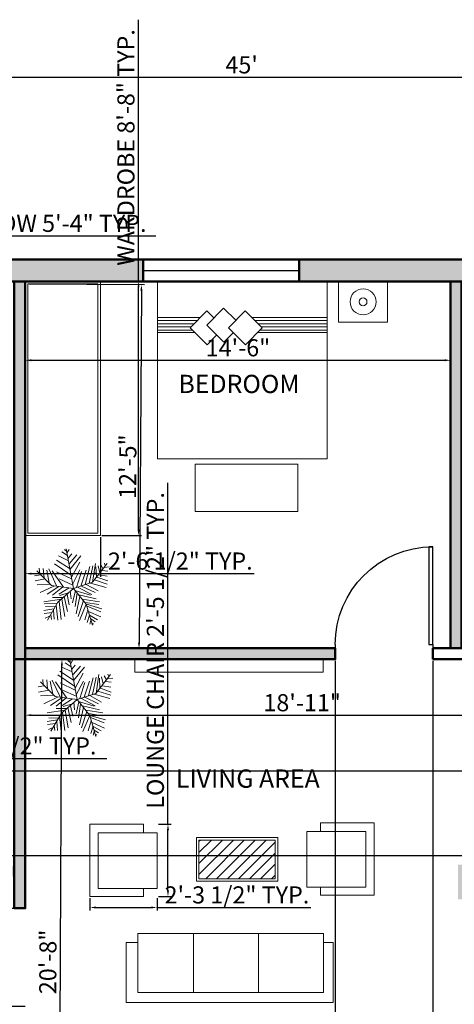
# Model space of a CAD drawing. Units: inches. Extents: x 1647 to 2354, y 1705 to 2321.
# Tile 3 of 4: x 1907 to 2085, y 1919 to 2321. Entities that reach past the tile are written whole.
import ezdxf

# ---------------------------------------------------------------- set-up
doc = ezdxf.new("R2010")
doc.units = ezdxf.units.IN
for name, color, linetype, lineweight in [('A-ANNO-DIMS', 130, 'Continuous', 18), ('A-AREA-IDEN', 7, 'Continuous', 25), ('A-FURN-PATT', 52, 'Continuous', 13), ('A-WALL-PATT', 84, 'Continuous', 13), ('door', 142, 'Continuous', 25), ('fur', 52, 'Continuous', 18), ('tree', 92, 'Continuous', 13), ('wall', 84, 'Continuous', 50), ('window', 242, 'Continuous', 25)]:
    doc.layers.add(name, color=color, linetype=linetype, lineweight=lineweight)
doc.styles.get("Standard").update_dxf_attribs({"font": 'arial.ttf'})
doc.dimstyles.new('ISO-25', dxfattribs={"dimtxt": 7, "dimasz": 2.5, "dimexe": 1.25, "dimexo": 0.625, "dimtad": 1, "dimdec": 0, "dimlunit": 4, "dimtxsty": 'Standard', "dimcen": 2.5, "dimadec": 0, "dimazin": 0, "dimtfac": 1, "dimtdec": 0, "dimtmove": 0, "dimatfit": 3, "dimfxl": 1, "dimarcsym": 0})

# ---------------------------------------------------------------- blocks, each defined once
blk = doc.blocks.new('*U2')
for p, q in [((0, 0), (0, -6)), ((40, 0), (40, -6))]:
    blk.add_line(p, q)
blk.add_lwpolyline([(0, 0), (0, 40), (1.75, 40), (1.75, 0)], close=True)
blk.add_arc((0, 0), 40, 0, 90)
blk = doc.blocks.new('*U6')
for p, q in [((0, 0), (-10.5, 57)), ((-7.288, 39.707), (-21.778, 46.673)), ((-8.737, 47.138), (-17.069, 52.711)), ((-10.186, 53.64), (-13.084, 55.962)), ((-9.099, 51.782), (-6.563, 55.962)), ((-7.65, 43.423), (-2.578, 49.46)), ((-5.839, 35.992), (4.667, 48.067)), ((-5.114, 27.632), (10.463, 46.673)), ((-48.585, 21.131), (-49.309, 29.026)), ((-43.513, 28.561), (-42.427, 15.558)), ((-3.665, 19.273), (-27.574, 35.527)), ((-5.114, 28.097), (-24.676, 40.636)), ((-2.941, 16.486), (8.652, 37.85)), ((16.259, 5.805), (23.142, 31.348)), ((22.055, 7.198), (27.489, 32.277)), ((27, 9), (48, 36)), ((27.127, 9.056), (31.112, 35.992)), ((31.836, 30.883), (32.561, 16.486)), ((35.096, 32.741), (37.27, 22.524)), ((38.719, 34.134), (41.979, 28.561)), ((43.791, 29.954), (51.036, 30.883)), ((44.153, 36.456), (45.239, 32.741)), ((-47.498, 19.737), (-55.83, 18.344)), ((-31.5, 4.5), (-52.5, 25.5)), ((-38.442, 26.239), (-34.819, 7.663)), ((-35.544, 28.097), (-24.314, 3.947)), ((-14.533, 2.09), (-30.834, 25.31)), ((-24.314, 23.917), (-2.941, 13.7)), ((-1.129, 6.734), (9.014, 26.704)), ((3.942, 1.625), (11.187, 24.381)), ((10.101, 3.483), (17.708, 26.239)), ((33.285, 16.486), (48.862, 10.913)), ((36.183, 19.737), (48.137, 17.88)), ((40.53, 25.775), (48.862, 24.846)), ((-40.615, 13.7), (-55.105, 10.913)), ((-33.37, 6.269), (-52.207, 5.34)), ((-28.299, 3.483), (-47.86, -5.805)), ((-21.416, 3.018), (-38.079, -8.128)), ((0, 0), (-31.5, 4.5)), ((-15.982, 2.09), (-30.11, -9.521)), ((0, 0), (-22.5, -19.5)), ((-6.563, 1.161), (-21.416, -8.128)), ((-20.691, 13.7), (-1.129, 4.876)), ((0, 0), (27, 9)), ((0, 0), (18, -22.5)), ((6.478, 1.625), (26.04, -8.592)), ((11.187, 3.483), (30.749, -5.805)), ((18.07, 5.805), (35.096, -3.483)), ((24.229, 7.663), (46.688, 1.625)), ((29.662, 12.307), (48.137, 6.269)), ((-15.257, -12.772), (-30.11, -12.772)), ((-6.563, -5.805), (-19.967, -9.985)), ((-13.446, -11.378), (-8.737, -32.741)), ((-9.461, -8.592), (-6.201, -23.453)), ((-4.752, -3.483), (-3.665, -14.629)), ((2.493, -3.019), (-1.491, -20.202)), ((1.769, -2.555), (24.229, -9.521)), ((5.029, -6.27), (2.131, -25.775)), ((9.014, -11.378), (3.58, -35.992)), ((7.565, -9.056), (32.198, -14.629)), ((-17.431, -15.094), (-42.789, -18.809)), ((-24.314, -21.596), (-42.427, -22.06)), ((-26.849, -26.24), (-40.253, -25.775)), ((-22.5, -19.5), (-37.5, -45)), ((-25.038, -23.918), (-22.865, -45.281)), ((-20.691, -18.345), (-17.793, -44.352)), ((-17.069, -15.094), (-12.721, -40.172)), ((14.085, -16.951), (6.478, -40.172)), ((18.07, -22.524), (8.289, -45.745)), ((12.274, -15.094), (36.907, -18.809)), ((16.259, -19.738), (36.183, -22.989)), ((18, -22.5), (27, -52.5)), ((18.433, -22.524), (40.53, -29.026)), ((19.157, -25.311), (38.719, -33.206)), ((-28.299, -29.026), (-42.789, -31.348)), ((-30.834, -34.135), (-42.427, -35.528)), ((-34.457, -39.708), (-40.978, -42.494)), ((-32.646, -36.921), (-31.921, -44.352)), ((-29.023, -30.884), (-27.936, -43.887)), ((20.244, -30.419), (15.897, -44.816)), ((22.78, -37.85), (19.519, -48.532)), ((21.331, -32.741), (39.081, -40.636)), ((22.78, -38.314), (34.372, -44.816)), ((24.591, -45.745), (23.142, -50.854)), ((24.591, -43.423), (30.749, -47.603)), ((26.764, -49.925), (28.213, -50.854))]:
    blk.add_line(p, q)
blk = doc.blocks.new('*D9')
at = {"layer": 'A-ANNO-DIMS', "color": 0, "lineweight": -2, "transparency": 16777216}
for p, q in [((1909.63, 2213.61), (1909.63, 2180.71)), ((2083.63, 2213.61), (2083.63, 2180.71)), ((1912.13, 2181.96), (2081.13, 2181.96))]:
    blk.add_line(p, q, dxfattribs=at)
at = {"layer": 'A-ANNO-DIMS', "color": 0, "transparency": 16777216}
for points in [[(1912.13, 2182.38), (1912.13, 2181.54), (1909.63, 2181.96)], [(2081.13, 2182.38), (2081.13, 2181.54), (2083.63, 2181.96)]]:
    blk.add_solid(points, dxfattribs=at)
at = {"layer": 'Defpoints', "color": 0, "transparency": 16777216}
for p in [(1909.63, 2214.23), (2083.63, 2214.23), (2083.63, 2181.96)]:
    blk.add_point(p, dxfattribs=at)
at = {"layer": 'A-ANNO-DIMS', "color": 0, "transparency": 16777216, "insert": (1996.63, 2186.16), "char_height": 7, "attachment_point": 5}
blk.add_mtext('14\'-6"', dxfattribs=at)
blk = doc.blocks.new('*D10')
at = {"layer": 'A-ANNO-DIMS', "color": 0, "lineweight": -2, "transparency": 16777216}
for p, q in [((1911.26, 2213.23), (1958.39, 2212.91)), ((1957.12, 2210.42), (1956.15, 2066.42)), ((1910.26, 2064.23), (1957.39, 2063.91))]:
    blk.add_line(p, q, dxfattribs=at)
at = {"layer": 'A-ANNO-DIMS', "color": 0, "transparency": 16777216}
for points in [[(1956.7, 2210.42), (1957.54, 2210.42), (1957.14, 2212.92)], [(1955.74, 2066.42), (1956.57, 2066.42), (1956.14, 2063.92)]]:
    blk.add_solid(points, dxfattribs=at)
at = {"layer": 'Defpoints', "color": 0, "transparency": 16777216}
for p in [(1910.63, 2213.23), (1909.63, 2064.23), (1956.14, 2063.92)]:
    blk.add_point(p, dxfattribs=at)
at = {"layer": 'A-ANNO-DIMS', "color": 0, "transparency": 16777216, "insert": (1952.44, 2138.45), "char_height": 7, "attachment_point": 5, "rotation": 89.6155}
blk.add_mtext('12\'-5"', dxfattribs=at)
blk = doc.blocks.new('*D16')
at = {"layer": 'A-ANNO-DIMS', "color": 0, "lineweight": -2, "transparency": 16777216}
for p, q in [((1911.55, 2059.73), (1925.86, 2059.66)), ((1923.34, 1814.66), (1924.6, 2057.16)), ((1910.26, 1812.23), (1924.57, 1812.16))]:
    blk.add_line(p, q, dxfattribs=at)
at = {"layer": 'A-ANNO-DIMS', "color": 0, "transparency": 16777216}
for points in [[(1924.18, 2057.16), (1925.01, 2057.16), (1924.61, 2059.66)], [(1922.92, 1814.66), (1923.75, 1814.66), (1923.32, 1812.16)]]:
    blk.add_solid(points, dxfattribs=at)
at = {"layer": 'Defpoints', "color": 0, "transparency": 16777216}
for p in [(1910.92, 2059.73), (1924.61, 2059.66), (1909.63, 1812.23)]:
    blk.add_point(p, dxfattribs=at)
at = {"layer": 'A-ANNO-DIMS', "color": 0, "transparency": 16777216, "insert": (1919.77, 1935.93), "char_height": 7, "attachment_point": 5, "rotation": 89.702}
blk.add_mtext('20\'-8"', dxfattribs=at)
blk = doc.blocks.new('*D23')
at = {"layer": 'A-ANNO-DIMS', "color": 0, "lineweight": -2, "transparency": 16777216}
for p, q in [((1909.63, 2059.11), (1909.63, 2035.57)), ((2136.13, 2059.11), (2136.13, 2035.57)), ((1912.13, 2036.82), (2133.63, 2036.82))]:
    blk.add_line(p, q, dxfattribs=at)
at = {"layer": 'A-ANNO-DIMS', "color": 0, "transparency": 16777216}
for points in [[(1912.13, 2037.24), (1912.13, 2036.41), (1909.63, 2036.82)], [(2133.63, 2037.24), (2133.63, 2036.41), (2136.13, 2036.82)]]:
    blk.add_solid(points, dxfattribs=at)
at = {"layer": 'Defpoints', "color": 0, "transparency": 16777216}
for p in [(1909.63, 2059.73), (2136.13, 2059.73), (2136.13, 2036.82)]:
    blk.add_point(p, dxfattribs=at)
at = {"layer": 'A-ANNO-DIMS', "color": 0, "transparency": 16777216, "insert": (2022.88, 2041.02), "char_height": 7, "attachment_point": 5}
blk.add_mtext('18\'-11"', dxfattribs=at)
blk = doc.blocks.new('*D24')
at = {"layer": 'A-ANNO-DIMS', "color": 0, "lineweight": -2, "transparency": 16777216}
for p, q in [((1728.13, 2223.86), (1728.13, 2298.93)), ((1730.63, 2297.68), (2265.63, 2297.68)), ((2268.13, 2223.86), (2268.13, 2298.93))]:
    blk.add_line(p, q, dxfattribs=at)
at = {"layer": 'A-ANNO-DIMS', "color": 0, "transparency": 16777216}
for points in [[(1730.63, 2298.09), (1730.63, 2297.26), (1728.13, 2297.68)], [(2265.63, 2298.09), (2265.63, 2297.26), (2268.13, 2297.68)]]:
    blk.add_solid(points, dxfattribs=at)
at = {"layer": 'Defpoints', "color": 0, "transparency": 16777216}
for p in [(2268.13, 2297.68), (1728.13, 2223.23), (2268.13, 2223.23)]:
    blk.add_point(p, dxfattribs=at)
at = {"layer": 'A-ANNO-DIMS', "color": 0, "transparency": 16777216, "insert": (1998.13, 2301.86), "char_height": 7, "attachment_point": 5}
blk.add_mtext("45'", dxfattribs=at)
blk = doc.blocks.new('WIN-WIDE-9IN-WALL')
blk.add_line((0, 4.5), (63.83, 4.5))
blk.add_lwpolyline([(0, 9), (63.83, 9), (63.83, 0), (0, 0)], close=True)
blk = doc.blocks.new('WARDROBE-LONG')
for points in [[(0, 103.94), (30.72, 103.94), (30.72, 0), (0, 0)], [(1, 102.94), (29.72, 102.94), (29.72, 1), (1, 1)]]:
    blk.add_lwpolyline(points, close=True)
blk = doc.blocks.new('NIGHTSTAND-WITH-LAMP')
blk.add_lwpolyline([(0, 16.74), (20.08, 16.74), (20.08, 0), (0, 0)], close=True)
for radius in [5.31, 1.6]:
    blk.add_circle((10.04, 8.37), radius)
blk = doc.blocks.new('BED-PILLOW-AND-COVER-SET')
for p, q in [((0, 11.11), (17.43, 11.11)), ((0, 9.87), (16.21, 9.87)), ((0, 8.55), (14.92, 8.55)), ((38.64, 11.11), (69.38, 11.11)), ((39.89, 9.87), (69.38, 9.87)), ((41.22, 8.55), (69.38, 8.55)), ((0, 7.29), (13.67, 7.29)), ((0, 5.98), (14.28, 5.98)), ((0, 4.92), (15.36, 4.92)), ((31.01, 4.92), (31.05, 4.92)), ((40.88, 4.92), (69.38, 4.92)), ((41.93, 5.98), (69.38, 5.98)), ((42.51, 7.29), (69.38, 7.29))]:
    blk.add_line(p, q)
for points in [[(23.1, 10.95), (20.15, 13.86), (13.32, 6.93), (20.34, 0), (24.26, 3.97)], [(32.02, 9.99), (27.02, 14.92), (20.19, 7.99), (27.21, 1.06), (31.03, 4.93)]]:
    blk.add_lwpolyline(points)
blk.add_lwpolyline([(29.01, 6.93), (36.04, 0), (42.87, 6.93), (35.84, 13.86)], close=True)
blk = doc.blocks.new('BED-FOOT-BENCH')
blk.add_lwpolyline([(0, 19.36), (42.07, 19.36), (42.07, 0), (0, 0)], close=True)
blk = doc.blocks.new('LOUNGE-CHAIR')
for p, q in [((21.9, 29.65), (0, 29.65)), ((0, 29.65), (0, 0)), ((21.9, 26.08), (21.9, 29.65)), ((21.9, 0), (21.9, 3.27)), ((0, 0), (21.9, 0))]:
    blk.add_line(p, q)
blk.add_lwpolyline([(27.5, 26.08), (27.5, 3.27), (3.38, 3.27), (3.38, 26.08)], close=True)
blk = doc.blocks.new('*D35')
at = {"layer": 'A-ANNO-DIMS', "color": 0, "lineweight": -2, "transparency": 16777216}
for p, q in [((1778.6, 2223.86), (1778.6, 2234.06)), ((1781.1, 2232.81), (1839.94, 2232.81)), ((1842.44, 2223.86), (1842.44, 2234.06)), ((1842.44, 2232.81), (1963.01, 2232.81))]:
    blk.add_line(p, q, dxfattribs=at)
at = {"layer": 'A-ANNO-DIMS', "color": 0, "transparency": 16777216}
for points in [[(1781.1, 2233.22), (1781.1, 2232.39), (1778.6, 2232.81)], [(1839.94, 2233.22), (1839.94, 2232.39), (1842.44, 2232.81)]]:
    blk.add_solid(points, dxfattribs=at)
at = {"layer": 'Defpoints', "color": 0, "transparency": 16777216}
for p in [(1842.44, 2232.81), (1778.6, 2223.23), (1842.44, 2223.23)]:
    blk.add_point(p, dxfattribs=at)
at = {"layer": 'A-ANNO-DIMS', "color": 0, "transparency": 16777216, "insert": (1903.97, 2237.05), "char_height": 7, "attachment_point": 5}
blk.add_mtext('WIDE WINDOW 5\'-4" TYP.', dxfattribs=at)
blk = doc.blocks.new('*D45')
at = {"layer": 'A-ANNO-DIMS', "color": 0, "lineweight": -2, "transparency": 16777216}
for p, q in [((1955.95, 2214.23), (1955.95, 2321.24)), ((1940.98, 2214.23), (1957.2, 2214.23)), ((1955.95, 2112.79), (1955.95, 2211.73)), ((1940.98, 2110.29), (1957.2, 2110.29))]:
    blk.add_line(p, q, dxfattribs=at)
at = {"layer": 'A-ANNO-DIMS', "color": 0, "transparency": 16777216}
for points in [[(1955.53, 2211.73), (1956.36, 2211.73), (1955.95, 2214.23)], [(1955.53, 2112.79), (1956.36, 2112.79), (1955.95, 2110.29)]]:
    blk.add_solid(points, dxfattribs=at)
at = {"layer": 'Defpoints', "color": 0, "transparency": 16777216}
for p in [(1940.36, 2214.23), (1955.95, 2214.23), (1940.36, 2110.29)]:
    blk.add_point(p, dxfattribs=at)
at = {"layer": 'A-ANNO-DIMS', "color": 0, "transparency": 16777216, "insert": (1951.7, 2268.99), "char_height": 7, "attachment_point": 5, "rotation": 90}
blk.add_mtext('WARDROBE 8\'-8" TYP.', dxfattribs=at)
blk = doc.blocks.new('*D46')
at = {"layer": 'A-ANNO-DIMS', "color": 0, "lineweight": -2, "transparency": 16777216}
for p, q in [((1909.63, 2109.67), (1909.63, 2093.45)), ((1940.36, 2109.67), (1940.36, 2093.45)), ((1912.13, 2094.7), (1937.86, 2094.7)), ((1940.36, 2094.7), (2003.21, 2094.7))]:
    blk.add_line(p, q, dxfattribs=at)
at = {"layer": 'A-ANNO-DIMS', "color": 0, "transparency": 16777216}
for points in [[(1912.13, 2095.12), (1912.13, 2094.29), (1909.63, 2094.7)], [(1937.86, 2095.12), (1937.86, 2094.29), (1940.36, 2094.7)]]:
    blk.add_solid(points, dxfattribs=at)
at = {"layer": 'Defpoints', "color": 0, "transparency": 16777216}
for p in [(1909.63, 2110.29), (1940.36, 2110.29), (1940.36, 2094.7)]:
    blk.add_point(p, dxfattribs=at)
at = {"layer": 'A-ANNO-DIMS', "color": 0, "transparency": 16777216, "insert": (1973.03, 2098.95), "char_height": 7, "attachment_point": 5}
blk.add_mtext('2\'-6 1/2" TYP.', dxfattribs=at)
blk = doc.blocks.new('*D47')
at = {"layer": 'A-ANNO-DIMS', "color": 0, "lineweight": -2, "transparency": 16777216}
for p, q in [((1967.99, 1992.28), (1967.99, 2131.86)), ((1964.16, 1992.28), (1969.24, 1992.28)), ((1967.99, 1965.13), (1967.99, 1989.78)), ((1964.16, 1962.63), (1969.24, 1962.63))]:
    blk.add_line(p, q, dxfattribs=at)
at = {"layer": 'A-ANNO-DIMS', "color": 0, "transparency": 16777216}
for points in [[(1967.57, 1989.78), (1968.4, 1989.78), (1967.99, 1992.28)], [(1967.57, 1965.13), (1968.4, 1965.13), (1967.99, 1962.63)]]:
    blk.add_solid(points, dxfattribs=at)
at = {"layer": 'Defpoints', "color": 0, "transparency": 16777216}
for p in [(1963.54, 1992.28), (1967.99, 1992.28), (1963.54, 1962.63)]:
    blk.add_point(p, dxfattribs=at)
at = {"layer": 'A-ANNO-DIMS', "color": 0, "transparency": 16777216, "insert": (1963.74, 2063.32), "char_height": 7, "attachment_point": 5, "rotation": 90}
blk.add_mtext('LOUNGE CHAIR 2\'-5 1/2" TYP.', dxfattribs=at)
blk = doc.blocks.new('*D48')
at = {"layer": 'A-ANNO-DIMS', "color": 0, "lineweight": -2, "transparency": 16777216}
for p, q in [((1936.04, 1962), (1936.04, 1956.93)), ((1963.54, 1962), (1963.54, 1956.93)), ((1938.54, 1958.18), (1961.04, 1958.18)), ((1963.54, 1958.18), (2026.39, 1958.18))]:
    blk.add_line(p, q, dxfattribs=at)
at = {"layer": 'A-ANNO-DIMS', "color": 0, "transparency": 16777216}
for points in [[(1938.54, 1958.59), (1938.54, 1957.76), (1936.04, 1958.18)], [(1961.04, 1958.59), (1961.04, 1957.76), (1963.54, 1958.18)]]:
    blk.add_solid(points, dxfattribs=at)
at = {"layer": 'Defpoints', "color": 0, "transparency": 16777216}
for p in [(1936.04, 1962.63), (1963.54, 1962.63), (1963.54, 1958.18)]:
    blk.add_point(p, dxfattribs=at)
at = {"layer": 'A-ANNO-DIMS', "color": 0, "transparency": 16777216, "insert": (1996.21, 1962.42), "char_height": 7, "attachment_point": 5}
blk.add_mtext('2\'-3 1/2" TYP.', dxfattribs=at)
blk = doc.blocks.new('*D49')
at = {"layer": 'A-ANNO-DIMS', "color": 0, "lineweight": -2, "transparency": 16777216}
for p, q in [((1757.95, 2022.05), (1757.95, 2017.87)), ((1781.7, 2022.05), (1781.7, 2017.87)), ((1760.45, 2019.12), (1779.2, 2019.12)), ((1781.7, 2019.12), (1942.97, 2019.12))]:
    blk.add_line(p, q, dxfattribs=at)
at = {"layer": 'A-ANNO-DIMS', "color": 0, "transparency": 16777216}
for points in [[(1760.45, 2019.53), (1760.45, 2018.7), (1757.95, 2019.12)], [(1779.2, 2019.53), (1779.2, 2018.7), (1781.7, 2019.12)]]:
    blk.add_solid(points, dxfattribs=at)
at = {"layer": 'Defpoints', "color": 0, "transparency": 16777216}
for p in [(1757.95, 2022.68), (1781.7, 2022.68), (1781.7, 2019.12)]:
    blk.add_point(p, dxfattribs=at)
at = {"layer": 'A-ANNO-DIMS', "color": 0, "transparency": 16777216, "insert": (1863.58, 2023.36), "char_height": 7, "attachment_point": 5}
blk.add_mtext('DINING END CHAIR 1\'-11 1/2" TYP.', dxfattribs=at)
blk = doc.blocks.new('*D56')
at = {"layer": 'A-ANNO-DIMS', "color": 0, "lineweight": -2, "transparency": 16777216}
for p, q in [((2036.41, 2059.11), (2036.41, 1752.18)), ((2076.41, 2059.11), (2076.41, 1752.18)), ((2038.91, 1753.43), (2073.91, 1753.43))]:
    blk.add_line(p, q, dxfattribs=at)
at = {"layer": 'A-ANNO-DIMS', "color": 0, "transparency": 16777216}
for points in [[(2038.91, 1753.85), (2038.91, 1753.02), (2036.41, 1753.43)], [(2073.91, 1753.85), (2073.91, 1753.02), (2076.41, 1753.43)]]:
    blk.add_solid(points, dxfattribs=at)
at = {"layer": 'Defpoints', "color": 0, "transparency": 16777216}
for p in [(2036.41, 2059.73), (2076.41, 2059.73), (2076.41, 1753.43)]:
    blk.add_point(p, dxfattribs=at)
at = {"layer": 'A-ANNO-DIMS', "color": 0, "transparency": 16777216, "insert": (2056.41, 1757.63), "char_height": 7, "attachment_point": 5}
blk.add_mtext('3\'-4"', dxfattribs=at)
blk = doc.blocks.new('*D57')
at = {"layer": 'A-ANNO-DIMS', "color": 0, "lineweight": -2, "transparency": 16777216}
for p, q in [((2135.51, 2013.92), (1693.08, 2013.92)), ((1694.33, 2011.42), (1694.33, 1981.78)), ((2135.51, 1979.28), (1693.08, 1979.28)), ((1694.33, 1979.28), (1694.33, 1935.05))]:
    blk.add_line(p, q, dxfattribs=at)
at = {"layer": 'A-ANNO-DIMS', "color": 0, "transparency": 16777216}
for points in [[(1693.92, 2011.42), (1694.75, 2011.42), (1694.33, 2013.92)], [(1693.92, 1981.78), (1694.75, 1981.78), (1694.33, 1979.28)]]:
    blk.add_solid(points, dxfattribs=at)
at = {"layer": 'Defpoints', "color": 0, "transparency": 16777216}
for p in [(2136.13, 2013.92), (1694.33, 1979.28), (2136.13, 1979.28)]:
    blk.add_point(p, dxfattribs=at)
at = {"layer": 'A-ANNO-DIMS', "color": 0, "transparency": 16777216, "insert": (1690.09, 1955.92), "char_height": 7, "attachment_point": 5, "rotation": 90}
blk.add_mtext('2\'-10 1/2"', dxfattribs=at)

msp = doc.modelspace()

# ---------------------------------------------------------------- hatches: boundary and pattern name
at = {"layer": 'A-FURN-PATT'}
h = msp.add_hatch(dxfattribs=at)
h.set_pattern_fill('ANSI31', color=256)
h.paths.add_polyline_path([(2011.87, 1985.75), (1980.61, 1985.75), (1980.61, 1969.95), (2011.87, 1969.95)])
at = {"layer": 'A-WALL-PATT'}
h = msp.add_hatch(color=256, dxfattribs=at)
h.dxf.hatch_style = 1
h.paths.add_polyline_path([(1957.79, 2223.23), (1842.44, 2223.23), (1842.44, 2214.23), (1957.79, 2214.23)])
h.paths.add_polyline_path([(2147.66, 2223.23), (2021.62, 2223.23), (2021.62, 2214.23), (2147.66, 2214.23)])
h.paths.add_polyline_path([(2088.13, 2214.23), (2083.63, 2214.23), (2083.63, 2064.23), (2088.13, 2064.23)])
h.paths.add_polyline_path([(1909.63, 2214.23), (1905.13, 2214.23), (1905.13, 2059.73), (1909.63, 2059.73), (1909.63, 2064.23)])
h.paths.add_polyline_path([(1737.13, 2017.09), (1728.13, 2017.09), (1728.13, 1920.4), (1737.13, 1920.4)])
h.paths.add_polyline_path([(1905.13, 1975.23), (1737.13, 1975.23), (1737.13, 1970.73), (1905.13, 1970.73)])
h.paths.add_polyline_path([(1909.63, 2059.73), (1905.13, 2059.73), (1905.13, 1957.89), (1909.63, 1957.89)])
h.paths.add_polyline_path([(2036.41, 2064.23), (1909.63, 2064.23), (1909.63, 2059.73), (2036.41, 2059.73)])
h.paths.add_polyline_path([(2140.63, 1979.28), (2136.13, 1979.28), (2136.13, 1971.23), (2140.63, 1971.23)])
h.paths.add_polyline_path([(2136.13, 1975.73), (2091.13, 1975.73), (2091.13, 1971.23), (2136.13, 1971.23)])
h.paths.add_polyline_path([(2091.13, 1975.73), (2086.63, 1975.73), (2086.63, 1961.55), (2091.13, 1961.55)])
h.paths.add_polyline_path([(2259.13, 1975.73), (2140.63, 1975.73), (2140.63, 1971.23), (2259.13, 1971.23)])
h.paths.add_polyline_path([(2205.13, 2000.82), (2200.63, 2000.82), (2200.63, 1975.73), (2205.13, 1975.73)])
h.paths.add_polyline_path([(2268.13, 2111.84), (2259.13, 2111.84), (2259.13, 2036.03), (2268.13, 2036.03)])
h.paths.add_polyline_path([(2259.13, 2064.23), (2240.73, 2064.23), (2240.73, 2059.73), (2259.13, 2059.73)])
h.paths.add_polyline_path([(2268.13, 1998.35), (2259.13, 1998.35), (2259.13, 1989.23), (2259.13, 1920.66), (2268.13, 1920.66)])

# ---------------------------------------------------------------- linework, layer by layer
at = {"layer": 'fur'}
for p, q in [((1978.44, 1947.56), (1978.44, 1923.43)), ((2005.02, 1947.56), (2005.02, 1923.43)), ((1955.63, 1943.85), (1950.9, 1943.85)), ((1950.9, 1943.85), (1950.9, 1919.29)), ((1955.63, 1943.85), (1955.63, 1943.85)), ((2035.59, 1943.85), (2031.66, 1943.85)), ((2035.59, 1919.29), (2035.59, 1943.85)), ((1950.9, 1919.29), (2035.59, 1919.29))]:
    msp.add_line(p, q, dxfattribs=at)
msp.add_lwpolyline([(2021.62, 2214.23), (2033.08, 2214.23), (2033.08, 2141.71), (1963.7, 2141.71), (1963.7, 2214.23)], dxfattribs=at)
for points in [[(1954.39, 2059.73), (2031.52, 2059.73), (2031.52, 2054.47), (1954.39, 2054.47)], [(1979.61, 1986.75), (2012.87, 1986.75), (2012.87, 1968.95), (1979.61, 1968.95)], [(1980.61, 1985.75), (2011.87, 1985.75), (2011.87, 1969.95), (1980.61, 1969.95)], [(1955.63, 1923.43), (2031.66, 1923.43), (2031.66, 1947.56), (1955.63, 1947.56)], [(1955.63, 1947.56), (1978.44, 1947.56), (1978.44, 1923.43), (1955.63, 1923.43)]]:
    msp.add_lwpolyline(points, close=True, dxfattribs=at)
at = {"layer": 'wall'}
for p, q in [((1728.13, 2223.23), (2268.13, 2223.23)), ((1909.63, 2214.23), (1909.63, 2064.23)), ((1909.63, 2214.23), (2083.63, 2214.23)), ((2083.63, 2214.23), (2083.63, 2064.23)), ((2036.41, 2064.23), (1909.63, 2064.23)), ((2083.63, 2064.23), (2076.41, 2064.23)), ((1909.63, 2059.73), (1909.63, 1970.73)), ((2036.41, 2059.73), (1909.63, 2059.73)), ((2088.13, 2059.73), (2076.41, 2059.73)), ((1909.63, 1970.73), (1909.63, 1957.89))]:
    msp.add_line(p, q, dxfattribs=at)
for points in [[(2101.16, 1803.23), (1728.13, 1803.23), (1728.13, 2223.23), (2268.13, 2223.23), (2268.13, 1803.23), (2159.48, 1803.23)], [(1909.63, 2214.23), (2083.63, 2214.23)]]:
    msp.add_lwpolyline(points, dxfattribs=at)
for points in [[(1842.44, 2223.23), (1957.79, 2223.23), (1957.79, 2214.23), (1842.44, 2214.23)], [(2021.62, 2214.23), (2147.66, 2214.23), (2147.66, 2223.23), (2021.62, 2223.23)], [(1905.13, 2214.23), (1909.63, 2214.23), (1909.63, 2059.73), (1905.13, 2059.73)], [(2083.63, 2064.23), (2088.13, 2064.23), (2088.13, 2214.23), (2083.63, 2214.23)], [(1909.63, 2064.23), (2036.41, 2064.23), (2036.41, 2059.73), (1909.63, 2059.73)], [(2076.41, 2059.73), (2093.85, 2059.73), (2093.85, 2064.23), (2076.41, 2064.23)], [(1905.13, 1957.89), (1909.63, 1957.89), (1909.63, 2059.73), (1905.13, 2059.73)]]:
    msp.add_lwpolyline(points, close=True, dxfattribs=at)

# ---------------------------------------------------------------- block references
at = {"layer": 'door', "xscale": -1}
msp.add_blockref('*U2', (2076.41, 2065.73), dxfattribs=at)
at = {"layer": 'door', "xscale": -1, "rotation": 90}
msp.add_blockref('*U2', (1903.63, 1957.89), dxfattribs=at)
at = {"layer": 'fur'}
for name, p in [('WARDROBE-LONG', (1909.63, 2110.29)), ('NIGHTSTAND-WITH-LAMP', (2037.77, 2197.49)), ('BED-PILLOW-AND-COVER-SET', (1963.7, 2188.34)), ('BED-FOOT-BENCH', (1979.05, 2120.11)), ('LOUNGE-CHAIR', (1936.04, 1962.63))]:
    msp.add_blockref(name, p, dxfattribs=at)
at = {"layer": 'fur', "extrusion": (0, 0, -1), "zscale": -1}
msp.add_blockref('LOUNGE-CHAIR', (-2052.28, 1963.19), dxfattribs=at)
at = {"layer": 'tree', "xscale": 0.2858091163346259, "yscale": 0.2858091163346259, "zscale": 0.2858091163346259}
for p in [(1929.4, 2088.61), (1930.82, 2043.17)]:
    msp.add_blockref('*U6', p, dxfattribs=at)
at = {"layer": 'window'}
msp.add_blockref('WIN-WIDE-9IN-WALL', (1957.79, 2214.23), dxfattribs=at)

# ---------------------------------------------------------------- texts
at = {"layer": 'A-AREA-IDEN', "attachment_point": 1}
for s, insert, char_height in [('BEDROOM', (1972.28, 2176.02), 7.465), ('LIVING AREA', (1971.22, 2014.63), 7.4646)]:
    msp.add_mtext_dynamic_manual_height_columns(s, width=263.8302, gutter_width=37.32, heights=[0], dxfattribs=dict(at, insert=insert, char_height=char_height))

# ---------------------------------------------------------------- dimensions: what is measured, and where the dimension line sits
at = {"layer": 'A-ANNO-DIMS'}
for base, p1, p2, text, picture, middle in [((1955.95, 2214.23), (1940.36, 2110.29), (1940.36, 2214.23), 'WARDROBE <> TYP.', '*D45', (1951.7, 2268.99)), ((1967.9872, 1992.2783), (1963.5393, 1962.6257), (1963.5393, 1992.2783), 'LOUNGE CHAIR <> TYP.', '*D47', (1963.7404, 2063.3167))]:
    dim = msp.add_linear_dim(base=base, p1=p1, p2=p2, angle=90, text=text, dimstyle='ISO-25', override={"dimdec": 1, "dimlfac": 1, "dimrnd": 0, "dimzin": 1, "dimdsep": 46, "dimlunit": 4, "dimfrac": 2}, dxfattribs=at)
    dim.commit()
    dim.dimension.update_dxf_attribs({"geometry": picture, "text_midpoint": middle})
for base, p1, p2, override, picture, middle in [((2268.13, 2297.68), (1728.13, 2223.23), (2268.13, 2223.23), {"dimclrd": 0, "dimclre": 0, "dimclrt": 0}, '*D24', (1998.13, 2301.86)), ((2083.63, 2181.96), (1909.63, 2214.23), (2083.63, 2214.23), {"dimclrd": 0, "dimclre": 0, "dimclrt": 0}, '*D9', (1996.63, 2186.16)), ((2136.13438186, 2036.82443058), (1909.63438186, 2059.73275818), (2136.13438186, 2059.73275818), {"dimclrd": 0, "dimclre": 0, "dimclrt": 0}, '*D23', (2022.88438186, 2041.02344149)), ((2076.41, 1753.43), (2036.41, 2059.73), (2076.41, 2059.73), {"dimdec": 1, "dimlfac": 1, "dimrnd": 0, "dimzin": 1, "dimdsep": 46, "dimlunit": 4, "dimfrac": 2}, '*D56', (2056.41, 1757.63))]:
    dim = msp.add_linear_dim(base=base, p1=p1, p2=p2, dimstyle='ISO-25', override=override, dxfattribs=at)
    dim.commit()
    dim.dimension.update_dxf_attribs({"geometry": picture, "text_midpoint": middle})
for base, p1, p2, text, picture, middle in [((1842.44, 2232.81), (1778.6, 2223.23), (1842.44, 2223.23), 'WIDE WINDOW <> TYP.', '*D35', (1903.97, 2237.05)), ((1940.36, 2094.7), (1909.63, 2110.29), (1940.36, 2110.29), '<> TYP.', '*D46', (1973.03, 2098.95)), ((1781.6967, 2019.1164), (1757.952, 2022.6781), (1781.6967, 2022.6781), 'DINING END CHAIR <> TYP.', '*D49', (1863.5812, 2023.3608)), ((1963.54, 1958.18), (1936.04, 1962.63), (1963.54, 1962.63), '<> TYP.', '*D48', (1996.21, 1962.42))]:
    dim = msp.add_linear_dim(base=base, p1=p1, p2=p2, text=text, dimstyle='ISO-25', override={"dimdec": 1, "dimlfac": 1, "dimrnd": 0, "dimzin": 1, "dimdsep": 46, "dimlunit": 4, "dimfrac": 2}, dxfattribs=at)
    dim.commit()
    dim.dimension.update_dxf_attribs({"geometry": picture, "text_midpoint": middle})
for p1, p2, distance, picture, middle in [((1910.63, 2213.23), (1909.63, 2064.23), 46.5, '*D10', (1952.44, 2138.45)), ((1909.63, 1812.23), (1910.92, 2059.73), -13.69, '*D16', (1919.77, 1935.93))]:
    dim = msp.add_aligned_dim(p1=p1, p2=p2, distance=distance, dimstyle='ISO-25', override={"dimclrd": 0, "dimclre": 0, "dimclrt": 0}, dxfattribs=at)
    dim.commit()
    dim.dimension.update_dxf_attribs({"geometry": picture, "text_midpoint": middle})
dim = msp.add_linear_dim(base=(1694.33, 1979.28), p1=(2136.13, 2013.92), p2=(2136.13, 1979.28), angle=90, dimstyle='ISO-25', override={"dimdec": 1, "dimlfac": 1, "dimrnd": 0, "dimzin": 1, "dimdsep": 46, "dimlunit": 4, "dimfrac": 2}, dxfattribs=at)
dim.commit()
dim.dimension.update_dxf_attribs({"geometry": '*D57', "text_midpoint": (1690.09, 1955.92)})

doc.saveas('drawing.dxf')
